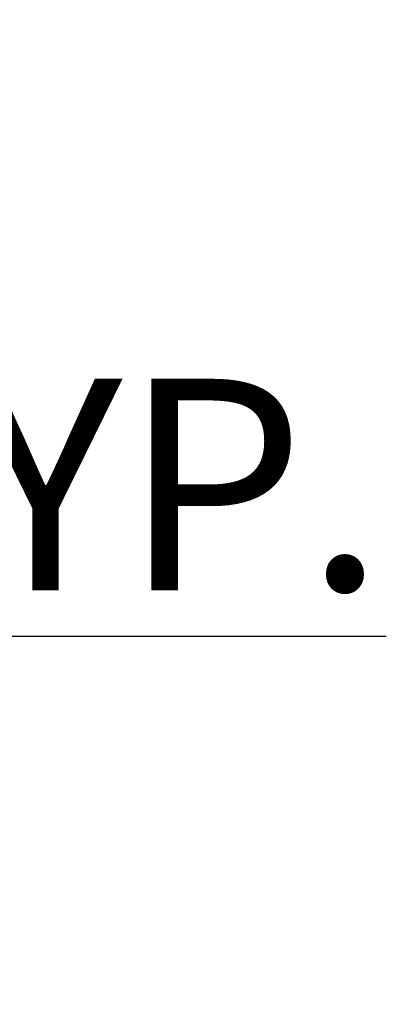
# Model space of a CAD drawing. Units: inches. Extents: x 3592 to 4861, y 1650 to 2243.
# Tile 6 of 30: x 4148 to 4164, y 1922 to 1964. Entities that reach past the tile are written whole.
import ezdxf

# ---------------------------------------------------------------- set-up
doc = ezdxf.new("R2010")
doc.units = ezdxf.units.IN
doc.layers.add('A-ANNO-DIMS', color=2, linetype='Continuous', lineweight=13)
doc.styles.get("Standard").update_dxf_attribs({"font": 'arial.ttf'})
doc.dimstyles.new('ISO-25', dxfattribs={"dimtxt": 9, "dimasz": 2.5, "dimexe": 1.25, "dimexo": 0.625, "dimtad": 1, "dimlunit": 3, "dimtxsty": 'Standard', "dimcen": 2.5, "dimadec": 0, "dimazin": 0, "dimtfac": 1, "dimtmove": 0, "dimatfit": 3, "dimfxl": 1, "dimarcsym": 0})

# ---------------------------------------------------------------- blocks, each defined once
blk = doc.blocks.new('*D153')
at = {"layer": 'A-ANNO-DIMS', "color": 0, "lineweight": -2, "transparency": 16777216}
for p, q in [((4066.445, 1941.594), (4066.445, 1936.486)), ((4085.182, 1941.594), (4085.182, 1936.486)), ((4068.945, 1937.736), (4082.682, 1937.736)), ((4085.182, 1937.736), (4163.916, 1937.736))]:
    blk.add_line(p, q, dxfattribs=at)
at = {"layer": 'A-ANNO-DIMS', "color": 0, "transparency": 16777216}
for points in [[(4068.945, 1938.153), (4068.945, 1937.319), (4066.445, 1937.736)], [(4082.682, 1938.153), (4082.682, 1937.319), (4085.182, 1937.736)]]:
    blk.add_solid(points, dxfattribs=at)
at = {"layer": 'Defpoints', "color": 0, "transparency": 16777216}
for p in [(4066.445, 1942.219), (4085.182, 1942.219), (4085.182, 1937.736)]:
    blk.add_point(p, dxfattribs=at)
at = {"layer": 'A-ANNO-DIMS', "color": 0, "transparency": 16777216, "insert": (4125.799, 1943.014), "char_height": 9, "attachment_point": 5}
blk.add_mtext('1\'-6 1/2" TYP.', dxfattribs=at)

msp = doc.modelspace()

# ---------------------------------------------------------------- dimensions: what is measured, and where the dimension line sits
at = {"layer": 'A-ANNO-DIMS'}
dim = msp.add_linear_dim(base=(4085.182, 1937.736), p1=(4066.445, 1942.219), p2=(4085.182, 1942.219), text='<> TYP.', dimstyle='ISO-25', override={"dimdec": 1, "dimlfac": 1, "dimrnd": 0, "dimzin": 1, "dimdsep": 46, "dimlunit": 4, "dimfrac": 2}, dxfattribs=at)
dim.commit()
dim.dimension.update_dxf_attribs({"geometry": '*D153', "text_midpoint": (4125.799, 1943.014)})

doc.saveas('drawing.dxf')
